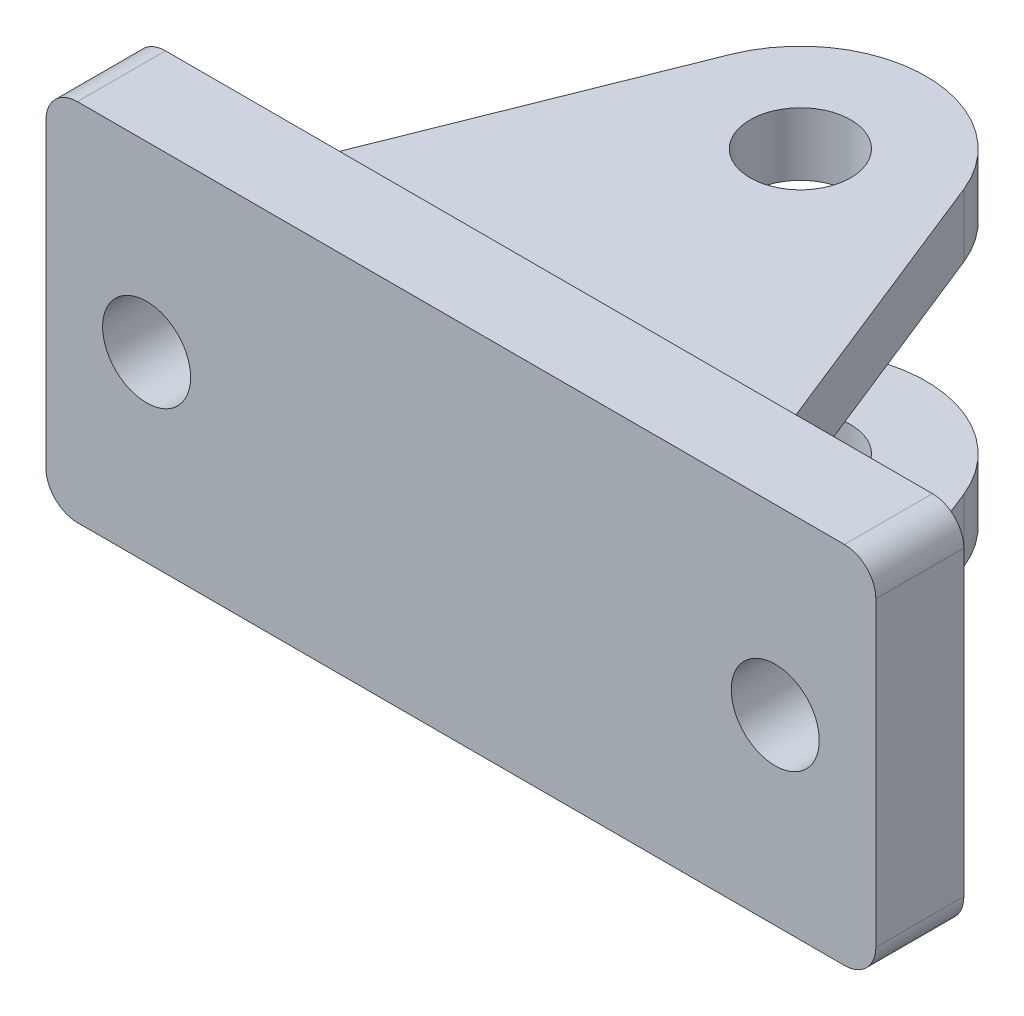
SolidWorks part; units mm, degrees
material "Plain Carbon Steel"
ref_plane "Front Plane" through (0, 0, 0) normal (0, 0, 1) x (1, 0, 0)
ref_plane "Top Plane" through (0, 0, 0) normal (0, 1, 0) x (1, 0, 0)
ref_plane "Right Plane" through (0, 0, 0) normal (1, 0, 0) x (0, 0, -1)
sketch "Base Plate Sketch" plane through (0, 0, 0) normal (0, 0, 1) x (1, 0, 0)
  line L0 (0, 96.1463) -> (0, -98.3287) construction
  line L1 (167.8013, 0) -> (-148.6448, 0) construction
  line L3 (-61, 29) -> (61, 29)
  line L4 (-66, 24) -> (-66, -24)
  line L5 (-61, -29) -> (61, -29)
  line L6 (66, 24) -> (66, -24)
  line L7 (-66, 29) -> (66, -29) construction
  line L8 (-66, -29) -> (66, 29) construction
  arc A0 (-66, 24) -> (-61, 29) centre (-61, 24) cw
  arc A1 (61, 29) -> (66, 24) centre (61, 24) cw
  arc A2 (61, -29) -> (66, -24) centre (61, -24) ccw
  arc A3 (-61, -29) -> (-66, -24) centre (-61, -24) cw
  circle A4 centre (-50, 0) radius 7
  circle A5 centre (50, 0) radius 7
  point P5 (0, 0)
  dimension "D3" = 5
  dimension "D1" = 14
  dimension "D2" = 100
  dimension "D4" = 16
  dimension "D5" = 29
extrude "Base Plate" add sketch "Base Plate Sketch" along normal blind 14
ref_plane "Lug Plane" through (0, 16, 0) normal (0, 1, 0) x (1, 0, 0)
sketch "Pivot Lug Sketch" plane through (0, 16, 0) normal (0, 1, 0) x (1, 0, 0)
  line L0 (0, -32.1909) -> (0, 54.0204) construction
  line L1 (61, -14) -> (-61, -14) construction
  line L2 (-37.5, 0) -> (37.5, 0)
  line L3 (61, 0) -> (-61, 0) construction
  line L4 (-37.5, 0) -> (-18.575, 47.4141)
  line L5 (37.5, 0) -> (18.575, 47.4141)
  circle A0 centre (0, 40) radius 8
  arc A1 (18.575, 47.4141) -> (-18.575, 47.4141) centre (0, 40) ccw
  dimension "D2" = 40
  dimension "D3" = 16
  dimension "D1" = 54
  dimension "D4" = 75
extrude "Pivot Lug" add sketch "Pivot Lug Sketch" along normal blind 10
mirror "Pivot Lug Mirror" about plane through (0, 0, 0) normal (0, 1, 0) of "Pivot Lug"
